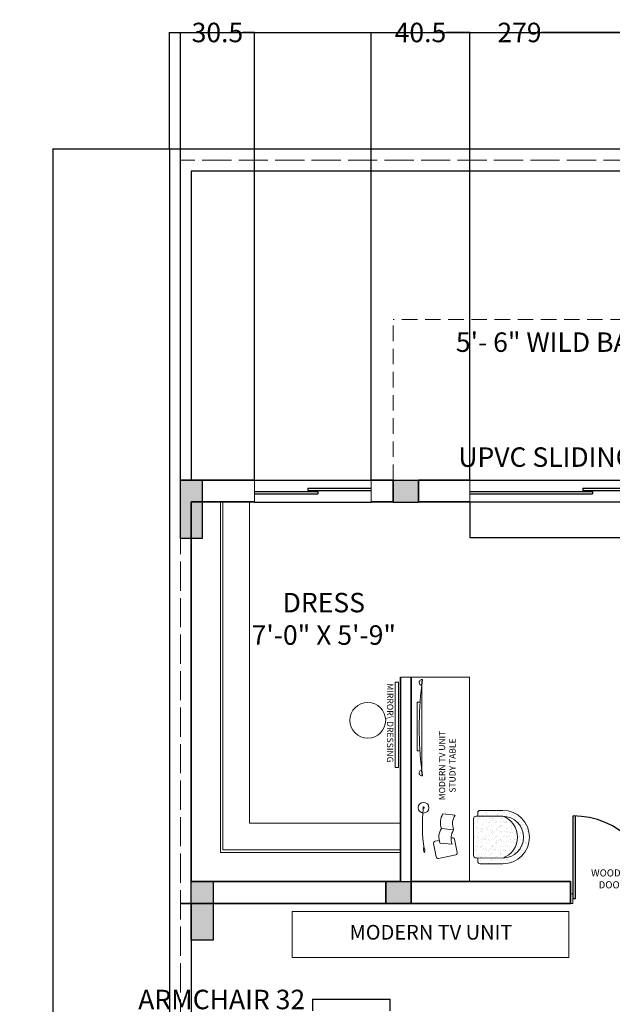
# Model space of a CAD drawing. Units: inches. Extents: x -48 to 50072, y 0 to 21068.
# Tile 54 of 75: x -48 to 196, y 819 to 1224. Entities that reach past the tile are written whole.
import ezdxf

# ---------------------------------------------------------------- set-up
doc = ezdxf.new("R2010")
doc.units = ezdxf.units.IN
doc.header["$MEASUREMENT"] = 0
doc.linetypes.add('ACAD_ISO02W100', pattern=[15, 12, -3])
doc.linetypes.add('HIDDEN', pattern=[9.525, 6.35, -3.175])
for name, color, linetype, lineweight in [('A-ANNO-DIMS', 2, 'Continuous', 18), ('A-ANNO-TEXT', 7, 'Continuous', 18), ('A-AREA-IDEN', 7, 'Continuous', 18), ('A-COLS', 1, 'Continuous', 35), ('A-DOOR', 4, 'Continuous', 18), ('A-EQPM', 8, 'Continuous', 18), ('A-FLOR-CASE', 9, 'Continuous', 18), ('A-FLOR-OVHD', 8, 'HIDDEN', 13), ('A-GLAZ', 4, 'Continuous', 18), ('A-WALL', 7, 'Continuous', 35), ('C-PROP', 7, 'Continuous', 25), ('C-PROP-REF', 32, 'ACAD_ISO02W100', 13), ('FURNITURE', 44, 'Continuous', 18)]:
    doc.layers.add(name, color=color, linetype=linetype, lineweight=lineweight)
doc.layers.add('Layer3', color=176, linetype='Continuous')
doc.styles.get("Standard").update_dxf_attribs({"font": 'arial.ttf'})
doc.dimstyles.get("Standard").update_dxf_attribs({"dimtxt": 8, "dimasz": 0.18, "dimexe": 0.18, "dimexo": 0.0625, "dimgap": 0.09, "dimtad": 0, "dimtih": 1, "dimtoh": 1, "dimdec": 1, "dimzin": 0, "dimdsep": 46, "dimlunit": 4, "dimtxsty": 'Standard', "dimblk": 'ARCHTICK', "dimcen": 0.09, "dimadec": 0, "dimazin": 0, "dimtfac": 1, "dimtdec": 1, "dimtofl": 0, "dimtmove": 0, "dimatfit": 3, "dimldrblk": 'ARCHTICK', "dimfxl": 1, "dimtolj": 1, "dimtzin": 0, "dimarcsym": 0})

# ---------------------------------------------------------------- blocks, each defined once
blk = doc.blocks.new('BKUHJKKUG')
at = {"layer": 'Defpoints'}
for p, q in [((179.52, 862.77), (179.52, 896.77)), ((180.52, 862.77), (180.52, 896.76)), ((179.52, 862.77), (180.52, 862.77))]:
    blk.add_line(p, q, dxfattribs=at)
blk.add_arc((179.52, 862.77), 34, 0, 90, dxfattribs=at)
at = {"insert": (190.84, 874.8), "char_height": 2.9183, "attachment_point": 1}
blk.add_mtext_dynamic_manual_height_columns('\\pxqc;WOODEN ^JDOOR', width=9.6242, gutter_width=14.59, heights=[0], dxfattribs=at)
blk = doc.blocks.new('khll')
at = {"layer": 'Defpoints'}
h = blk.add_hatch(color=256, dxfattribs=at)
h.dxf.hatch_style = 1
h.paths.add_polyline_path([(105.52, 1025.77), (116.02, 1025.77), (116.02, 1034.77), (105.52, 1034.77)])
for p, q in [((105.52, 1025.77), (105.52, 1034.77)), ((116.02, 1025.77), (116.02, 1034.77))]:
    blk.add_line(p, q)
for p, q in [((105.52, 1034.77), (116.02, 1034.77)), ((105.52, 1025.77), (116.02, 1025.77))]:
    blk.add_line(p, q, dxfattribs=at)
blk = doc.blocks.new('bnniku')
at = {"layer": 'Defpoints'}
h = blk.add_hatch(color=256, dxfattribs=at)
h.dxf.hatch_style = 1
h.paths.add_polyline_path([(767.55, 1114.04), (758.55, 1114.04), (758.55, 1090.04), (767.55, 1090.04)])
for p, q in [((758.55, 1114.04), (767.55, 1114.04)), ((758.55, 1090.04), (758.55, 1114.04)), ((767.55, 1114.04), (767.55, 1090.04)), ((767.55, 1090.04), (758.55, 1090.04))]:
    blk.add_line(p, q, dxfattribs=at)
blk = doc.blocks.new('windom')
for p, q in [((48.52, 1025.77), (48.52, 1034.77)), ((96.52, 1025.77), (96.52, 1034.77))]:
    blk.add_line(p, q)
at = {"layer": 'Defpoints'}
for p, q in [((48.52, 1030.07), (74.52, 1030.07)), ((48.52, 1029.07), (74.52, 1029.07)), ((70.52, 1031.47), (96.52, 1031.47)), ((70.52, 1031.47), (70.52, 1030.47)), ((70.52, 1030.47), (96.52, 1030.47)), ((74.52, 1030.07), (74.52, 1029.07))]:
    blk.add_line(p, q, dxfattribs=at)
at = {"layer": 'Layer3'}
for p, q in [((48.52, 1034.77), (96.52, 1034.77)), ((48.52, 1025.77), (96.52, 1025.77))]:
    blk.add_line(p, q, dxfattribs=at)
blk = doc.blocks.new('sliding')
blk.add_line((137.02, 1025.77), (137.02, 1034.77))
at = {"layer": 'Defpoints'}
for p, q in [((234.12, 1034.77), (234.12, 1025.77)), ((137.02, 1030.07), (187.57, 1030.07)), ((137.02, 1029.07), (187.57, 1029.07)), ((183.57, 1031.47), (234.12, 1031.47)), ((183.57, 1031.47), (183.57, 1030.47)), ((183.57, 1030.47), (234.12, 1030.47)), ((187.57, 1030.07), (187.57, 1029.07))]:
    blk.add_line(p, q, dxfattribs=at)
at = {"layer": 'Layer3'}
for p, q in [((137.02, 1034.77), (234.12, 1034.77)), ((234.12, 1025.77), (137.02, 1025.77))]:
    blk.add_line(p, q, dxfattribs=at)
blk = doc.blocks.new('CHAIR-STUDY')
for p, q in [((1.73, 20.94), (1.73, 19.57)), ((1.74, 20.38, 13.84), (1.74, 20.38, 13.84)), ((2.76, 21.97), (12.03, 21.96)), ((3.67, 21.9, 13.84), (3.67, 21.9, 13.84)), ((4.87, 21.05, 13.84), (4.87, 21.05, 13.84)), ((5.15, 21.3, 13.84), (5.15, 21.3, 13.84)), ((5.52, 20.9, 13.84), (5.52, 20.9, 13.84)), ((5.63, 20.39, 13.84), (5.63, 20.39, 13.84)), ((6.44, 21.95, 13.84), (6.44, 21.95, 13.84)), ((7.77, 21.75, 13.84), (7.77, 21.75, 13.84)), ((8.5, 21.68, 13.84), (8.5, 21.68, 13.84)), ((9.61, 20.34, 13.84), (9.61, 20.34, 13.84)), ((9.74, 21.52, 13.84), (9.74, 21.52, 13.84)), ((10.25, 20.89, 13.84), (10.25, 20.89, 13.84)), ((10.53, 21.41, 13.84), (10.53, 21.41, 13.84)), ((11.24, 21.36, 13.84), (11.24, 21.36, 13.84)), ((11.66, 21.77, 13.84), (11.66, 21.77, 13.84)), ((12.59, 21.14, 13.84), (12.59, 21.14, 13.84)), ((13.83, 20.98, 13.84), (13.83, 20.98, 13.84)), ((14.62, 20.87, 13.84), (14.62, 20.87, 13.84)), ((14.99, 20.88, 13.84), (14.99, 20.88, 13.84)), ((16.68, 20.6, 13.84), (16.68, 20.6, 13.84)), ((0.01, 18.54), (0, 3.44)), ((0.15, 18.84, 13.84), (0.15, 18.84, 13.84)), ((0.44, 16.98, 13.84), (0.44, 16.98, 13.84)), ((0.94, 18.74, 13.84), (0.94, 18.74, 13.84)), ((1.04, 19.57), (12.03, 19.56)), ((1.64, 17.45, 13.84), (1.64, 17.45, 13.84)), ((1.76, 18.19, 13.84), (1.76, 18.19, 13.84)), ((1.87, 18.57, 13.84), (1.87, 18.57, 13.84)), ((2.04, 18.45, 13.84), (2.04, 18.45, 13.84)), ((2.51, 18.98, 13.84), (2.51, 18.98, 13.84)), ((3.01, 18.47, 13.84), (3.01, 18.47, 13.84)), ((3.55, 19.84, 13.84), (3.55, 19.84, 13.84)), ((3.57, 18.97, 13.84), (3.57, 18.97, 13.84)), ((4.24, 18.3, 13.84), (4.24, 18.3, 13.84)), ((4.29, 17.09, 13.84), (4.29, 17.09, 13.84)), ((5.03, 18.2, 13.84), (5.03, 18.2, 13.84)), ((5.53, 17.47, 13.84), (5.53, 17.47, 13.84)), ((6.33, 16.86, 13.84), (6.33, 16.86, 13.84)), ((6.6, 18.56, 13.84), (6.6, 18.56, 13.84)), ((6.61, 17.12, 13.84), (6.61, 17.12, 13.84)), ((7.1, 17.93, 13.84), (7.1, 17.93, 13.84)), ((7.24, 18.97, 13.84), (7.24, 18.97, 13.84)), ((7.68, 18.82, 13.84), (7.68, 18.82, 13.84)), ((8.12, 18.5, 13.84), (8.12, 18.5, 13.84)), ((8.34, 17.77, 13.84), (8.34, 17.77, 13.84)), ((9.02, 17.09, 13.84), (9.02, 17.09, 13.84)), ((9.13, 17.66, 13.84), (9.13, 17.66, 13.84)), ((9.44, 19.71, 13.84), (9.44, 19.71, 13.84)), ((9.51, 17.42, 13.84), (9.51, 17.42, 13.84)), ((9.72, 19.97, 13.84), (9.72, 19.97, 13.84)), ((11.19, 17.39, 13.84), (11.19, 17.39, 13.84)), ((11.33, 18.56, 13.84), (11.33, 18.56, 13.84)), ((11.57, 18.84, 13.84), (11.57, 18.84, 13.84)), ((11.97, 18.96, 13.84), (11.97, 18.96, 13.84)), ((12.43, 17.23, 13.84), (12.43, 17.23, 13.84)), ((12.69, 17.17, 13.84), (12.69, 17.17, 13.84)), ((13.22, 17.12, 13.84), (13.22, 17.12, 13.84)), ((13.62, 17.27, 13.84), (13.62, 17.27, 13.84)), ((13.71, 20.2, 13.84), (13.71, 20.2, 13.84)), ((13.76, 17.08, 13.84), (13.76, 17.08, 13.84)), ((14.01, 18.38, 13.84), (14.01, 18.38, 13.84)), ((14.29, 18.64, 13.84), (14.29, 18.64, 13.84)), ((15.28, 16.85, 13.84), (15.28, 16.85, 13.84)), ((15.54, 18.79, 13.84), (15.54, 18.79, 13.84)), ((15.81, 20.02, 13.84), (15.81, 20.02, 13.84)), ((16.07, 18.55, 13.84), (16.07, 18.55, 13.84)), ((16.52, 16.69, 13.84), (16.52, 16.69, 13.84)), ((16.71, 18.96, 13.84), (16.71, 18.96, 13.84)), ((17.31, 16.58, 13.84), (17.31, 16.58, 13.84)), ((17.5, 17.29, 13.84), (17.5, 17.29, 13.84)), ((17.6, 20.21, 13.84), (17.6, 20.21, 13.84)), ((18.49, 17.07, 13.84), (18.49, 17.07, 13.84)), ((18.58, 17.05, 13.84), (18.58, 17.05, 13.84)), ((18.86, 17.3, 13.84), (18.86, 17.3, 13.84)), ((19.37, 16.31, 13.84), (19.37, 16.31, 13.84)), ((19.65, 18.64, 13.84), (19.65, 18.64, 13.84)), ((0.64, 14.77, 13.84), (0.64, 14.77, 13.84)), ((1.28, 15.17, 13.84), (1.28, 15.17, 13.84)), ((1.55, 14.52, 13.84), (1.55, 14.52, 13.84)), ((1.61, 14.72, 13.84), (1.61, 14.72, 13.84)), ((1.89, 12.79, 13.84), (1.89, 12.79, 13.84)), ((2.84, 14.55, 13.84), (2.84, 14.55, 13.84)), ((3.06, 13.29, 13.84), (3.06, 13.29, 13.84)), ((3.21, 14, 13.84), (3.21, 14, 13.84)), ((3.38, 13.11, 13.84), (3.38, 13.11, 13.84)), ((3.48, 16.04, 13.84), (3.48, 16.04, 13.84)), ((3.49, 14.26, 13.84), (3.49, 14.26, 13.84)), ((3.63, 14.45, 13.84), (3.63, 14.45, 13.84)), ((5.01, 15.65, 13.84), (5.01, 15.65, 13.84)), ((5.37, 14.76, 13.84), (5.37, 14.76, 13.84)), ((5.44, 14.54, 13.84), (5.44, 14.54, 13.84)), ((5.7, 14.18, 13.84), (5.7, 14.18, 13.84)), ((6.01, 15.17, 13.84), (6.01, 15.17, 13.84)), ((6.93, 14.01, 13.84), (6.93, 14.01, 13.84)), ((7.49, 12.96, 13.84), (7.49, 12.96, 13.84)), ((7.58, 15.89, 13.84), (7.58, 15.89, 13.84)), ((7.72, 13.91, 13.84), (7.72, 13.91, 13.84)), ((7.78, 12.67, 13.84), (7.78, 12.67, 13.84)), ((7.8, 13.28, 13.84), (7.8, 13.28, 13.84)), ((8.06, 12.93, 13.84), (8.06, 12.93, 13.84)), ((9.41, 14.49, 13.84), (9.41, 14.49, 13.84)), ((9.58, 14.31, 13.84), (9.58, 14.31, 13.84)), ((9.79, 13.64, 13.84), (9.79, 13.64, 13.84)), ((10.1, 14.75, 13.84), (10.1, 14.75, 13.84)), ((10.75, 15.16, 13.84), (10.75, 15.16, 13.84)), ((10.9, 15.52, 13.84), (10.9, 15.52, 13.84)), ((11.03, 13.48, 13.84), (11.03, 13.48, 13.84)), ((11.18, 15.78, 13.84), (11.18, 15.78, 13.84)), ((11.37, 12.98, 13.84), (11.37, 12.98, 13.84)), ((11.47, 15.91, 13.84), (11.47, 15.91, 13.84)), ((11.82, 13.37, 13.84), (11.82, 13.37, 13.84)), ((12.53, 13.27, 13.84), (12.53, 13.27, 13.84)), ((13.52, 14.34, 13.84), (13.52, 14.34, 13.84)), ((13.88, 13.1, 13.84), (13.88, 13.1, 13.84)), ((14.14, 12.98, 13.84), (14.14, 12.98, 13.84)), ((14.84, 14.74, 13.84), (14.84, 14.74, 13.84)), ((15.12, 12.94, 13.84), (15.12, 12.94, 13.84)), ((15.35, 12.93, 13.84), (15.35, 12.93, 13.84)), ((15.45, 15.86, 13.84), (15.45, 15.86, 13.84)), ((15.47, 14.19, 13.84), (15.47, 14.19, 13.84)), ((15.48, 15.15, 13.84), (15.48, 15.15, 13.84)), ((15.75, 14.45, 13.84), (15.75, 14.45, 13.84)), ((15.91, 12.83, 13.84), (15.91, 12.83, 13.84)), ((17.26, 15.83, 13.84), (17.26, 15.83, 13.84)), ((17.26, 13.26, 13.84), (17.26, 13.26, 13.84)), ((17.41, 14.36, 13.84), (17.41, 14.36, 13.84)), ((17.97, 12.56, 13.84), (17.97, 12.56, 13.84)), ((19.21, 12.4, 13.84), (19.21, 12.4, 13.84)), ((19.46, 12.78, 13.84), (19.46, 12.78, 13.84)), ((19.55, 15.71, 13.84), (19.55, 15.71, 13.84)), ((19.57, 14.73, 13.84), (19.57, 14.73, 13.84)), ((20, 12.29, 13.84), (20, 12.29, 13.84)), ((20.04, 12.86, 13.84), (20.04, 12.86, 13.84)), ((20.21, 15.14, 13.84), (20.21, 15.14, 13.84)), ((20.32, 13.11, 13.84), (20.32, 13.11, 13.84)), ((20.61, 16.15, 13.84), (20.61, 16.15, 13.84)), ((21.39, 14.31, 13.84), (21.39, 14.31, 13.84)), ((21.4, 16.05, 13.84), (21.4, 16.05, 13.84)), ((21.83, 14.5, 13.84), (21.83, 14.5, 13.84)), ((22, 13.25, 13.84), (22, 13.25, 13.84)), ((0.05, 11.37, 13.84), (0.05, 11.37, 13.84)), ((0.1, 11.15, 13.84), (0.1, 11.15, 13.84)), ((0.21, 10.96, 13.84), (0.21, 10.96, 13.84)), ((0.38, 11.41, 13.84), (0.38, 11.41, 13.84)), ((1.36, 8.66, 13.84), (1.36, 8.66, 13.84)), ((1.44, 10.8, 13.84), (1.44, 10.8, 13.84)), ((1.45, 11.59, 13.84), (1.45, 11.59, 13.84)), ((1.84, 9.48, 13.84), (1.84, 9.48, 13.84)), ((2.23, 10.7, 13.84), (2.23, 10.7, 13.84)), ((3.28, 10.18, 13.84), (3.28, 10.18, 13.84)), ((3.34, 8.6, 13.84), (3.34, 8.6, 13.84)), ((4.14, 10.95, 13.84), (4.14, 10.95, 13.84)), ((4.3, 10.43, 13.84), (4.3, 10.43, 13.84)), ((4.67, 9.81, 13.84), (4.67, 9.81, 13.84)), ((4.78, 11.36, 13.84), (4.78, 11.36, 13.84)), ((4.95, 10.07, 13.84), (4.95, 10.07, 13.84)), ((5.24, 8.68, 13.84), (5.24, 8.68, 13.84)), ((5.34, 11.61, 13.84), (5.34, 11.61, 13.84)), ((5.53, 10.26, 13.84), (5.53, 10.26, 13.84)), ((6.32, 10.16, 13.84), (6.32, 10.16, 13.84)), ((6.46, 11.46, 13.84), (6.46, 11.46, 13.84)), ((6.57, 9.47, 13.84), (6.57, 9.47, 13.84)), ((7.39, 10.04, 13.84), (7.39, 10.04, 13.84)), ((8.39, 9.89, 13.84), (8.39, 9.89, 13.84)), ((8.88, 10.94, 13.84), (8.88, 10.94, 13.84)), ((9.22, 8.63, 13.84), (9.22, 8.63, 13.84)), ((9.24, 8.48, 13.84), (9.24, 8.48, 13.84)), ((9.32, 11.56, 13.84), (9.32, 11.56, 13.84)), ((9.52, 11.35, 13.84), (9.52, 11.35, 13.84)), ((9.52, 8.74, 13.84), (9.52, 8.74, 13.84)), ((9.62, 9.72, 13.84), (9.62, 9.72, 13.84)), ((10.41, 9.62, 13.84), (10.41, 9.62, 13.84)), ((11.03, 10.12, 13.84), (11.03, 10.12, 13.84)), ((11.28, 10.05, 13.84), (11.28, 10.05, 13.84)), ((11.3, 9.46, 13.84), (11.3, 9.46, 13.84)), ((12.35, 11.34, 13.84), (12.35, 11.34, 13.84)), ((12.48, 9.35, 13.84), (12.48, 9.35, 13.84)), ((12.63, 11.59, 13.84), (12.63, 11.59, 13.84)), ((13.33, 8.48, 13.84), (13.33, 8.48, 13.84)), ((13.42, 11.41, 13.84), (13.42, 11.41, 13.84)), ((13.61, 10.93, 13.84), (13.61, 10.93, 13.84)), ((13.72, 9.19, 13.84), (13.72, 9.19, 13.84)), ((14.25, 11.34, 13.84), (14.25, 11.34, 13.84)), ((14.51, 9.08, 13.84), (14.51, 9.08, 13.84)), ((15.26, 10, 13.84), (15.26, 10, 13.84)), ((15.6, 8.79, 13.84), (15.6, 8.79, 13.84)), ((16.04, 9.46, 13.84), (16.04, 9.46, 13.84)), ((16.57, 8.81, 13.84), (16.57, 8.81, 13.84)), ((16.92, 10, 13.84), (16.92, 10, 13.84)), ((17.2, 10.26, 13.84), (17.2, 10.26, 13.84)), ((17.22, 8.5, 13.84), (17.22, 8.5, 13.84)), ((17.31, 11.43, 13.84), (17.31, 11.43, 13.84)), ((17.81, 8.65, 13.84), (17.81, 8.65, 13.84)), ((18.34, 10.93, 13.84), (18.34, 10.93, 13.84)), ((18.6, 8.54, 13.84), (18.6, 8.54, 13.84)), ((18.71, 11.64, 13.84), (18.71, 11.64, 13.84)), ((18.99, 11.33, 13.84), (18.99, 11.33, 13.84)), ((19.36, 9.86, 13.84), (19.36, 9.86, 13.84)), ((20.66, 8.27, 13.84), (20.66, 8.27, 13.84)), ((20.77, 9.45, 13.84), (20.77, 9.45, 13.84)), ((21.2, 8.45, 13.84), (21.2, 8.45, 13.84)), ((21.29, 11.38, 13.84), (21.29, 11.38, 13.84)), ((21.49, 8.67, 13.84), (21.49, 8.67, 13.84)), ((21.77, 8.92, 13.84), (21.77, 8.92, 13.84)), ((21.9, 8.11, 13.84), (21.9, 8.11, 13.84)), ((22.06, 12.02, 13.84), (22.06, 12.02, 13.84)), ((0.04, 7.05, 13.84), (0.04, 7.05, 13.84)), ((0.23, 5.75, 13.84), (0.23, 5.75, 13.84)), ((0.61, 5.68, 13.84), (0.61, 5.68, 13.84)), ((0.83, 6.95, 13.84), (0.83, 6.95, 13.84)), ((1.26, 5.73, 13.84), (1.26, 5.73, 13.84)), ((1.55, 6.96, 13.84), (1.55, 6.96, 13.84)), ((1.83, 7.22, 13.84), (1.83, 7.22, 13.84)), ((2.9, 6.68, 13.84), (2.9, 6.68, 13.84)), ((2.92, 7.15, 13.84), (2.92, 7.15, 13.84)), ((3.09, 4.33, 13.84), (3.09, 4.33, 13.84)), ((3.19, 7.25, 13.84), (3.19, 7.25, 13.84)), ((3.56, 7.55, 13.84), (3.56, 7.55, 13.84)), ((4.13, 6.51, 13.84), (4.13, 6.51, 13.84)), ((4.8, 4.41, 13.84), (4.8, 4.41, 13.84)), ((4.92, 6.41, 13.84), (4.92, 6.41, 13.84)), ((5.15, 5.75, 13.84), (5.15, 5.75, 13.84)), ((5.34, 5.67, 13.84), (5.34, 5.67, 13.84)), ((6.12, 5.63, 13.84), (6.12, 5.63, 13.84)), ((6.4, 5.88, 13.84), (6.4, 5.88, 13.84)), ((6.99, 6.14, 13.84), (6.99, 6.14, 13.84)), ((7.2, 4.18, 13.84), (7.2, 4.18, 13.84)), ((7.29, 7.11, 13.84), (7.29, 7.11, 13.84)), ((7.65, 7.14, 13.84), (7.65, 7.14, 13.84)), ((7.91, 7.27, 13.84), (7.91, 7.27, 13.84)), ((8.22, 5.97, 13.84), (8.22, 5.97, 13.84)), ((8.29, 7.55, 13.84), (8.29, 7.55, 13.84)), ((9.01, 5.87, 13.84), (9.01, 5.87, 13.84)), ((9.13, 5.7, 13.84), (9.13, 5.7, 13.84)), ((10.08, 5.66, 13.84), (10.08, 5.66, 13.84)), ((10.69, 4.29, 13.84), (10.69, 4.29, 13.84)), ((10.97, 4.55, 13.84), (10.97, 4.55, 13.84)), ((11.08, 5.6, 13.84), (11.08, 5.6, 13.84)), ((11.09, 4.2, 13.84), (11.09, 4.2, 13.84)), ((11.18, 7.13, 13.84), (11.18, 7.13, 13.84)), ((12.31, 5.44, 13.84), (12.31, 5.44, 13.84)), ((12.38, 7.13, 13.84), (12.38, 7.13, 13.84)), ((12.48, 5.93, 13.84), (12.48, 5.93, 13.84)), ((13.02, 7.54, 13.84), (13.02, 7.54, 13.84)), ((13.1, 5.33, 13.84), (13.1, 5.33, 13.84)), ((13.23, 5.55, 13.84), (13.23, 5.55, 13.84)), ((13.81, 7.15, 13.84), (13.81, 7.15, 13.84)), ((14.09, 7.4, 13.84), (14.09, 7.4, 13.84)), ((14.81, 5.65, 13.84), (14.81, 5.65, 13.84)), ((15.07, 4.15, 13.84), (15.07, 4.15, 13.84)), ((15.16, 7.07, 13.84), (15.16, 7.07, 13.84)), ((15.17, 5.06, 13.84), (15.17, 5.06, 13.84)), ((16.41, 4.9, 13.84), (16.41, 4.9, 13.84)), ((17.05, 4.6, 13.84), (17.05, 4.6, 13.84)), ((17.12, 7.12, 13.84), (17.12, 7.12, 13.84)), ((17.12, 5.57, 13.84), (17.12, 5.57, 13.84)), ((17.2, 4.79, 13.84), (17.2, 4.79, 13.84)), ((17.76, 7.53, 13.84), (17.76, 7.53, 13.84)), ((18.37, 5.81, 13.84), (18.37, 5.81, 13.84)), ((18.65, 6.07, 13.84), (18.65, 6.07, 13.84)), ((19.26, 4.52, 13.84), (19.26, 4.52, 13.84)), ((19.27, 6.93, 13.84), (19.27, 6.93, 13.84)), ((19.54, 5.64, 13.84), (19.54, 5.64, 13.84)), ((20.17, 7.46, 13.84), (20.17, 7.46, 13.84)), ((20.5, 4.36, 13.84), (20.5, 4.36, 13.84)), ((21.1, 5.52, 13.84), (21.1, 5.52, 13.84)), ((21.85, 7.11, 13.84), (21.85, 7.11, 13.84)), ((1.03, 2.41), (12.01, 2.4)), ((1.16, 2.8, 13.84), (1.16, 2.8, 13.84)), ((1.49, 2.92, 13.84), (1.49, 2.92, 13.84)), ((1.69, 3.34, 13.84), (1.69, 3.34, 13.84)), ((1.72, 2.41), (1.71, 1.04)), ((2.33, 3.75, 13.84), (2.33, 3.75, 13.84)), ((2.73, 2.76, 13.84), (2.73, 2.76, 13.84)), ((2.74, 0.01), (12.01, 0)), ((3, 1.4, 13.84), (3, 1.4, 13.84)), ((3.01, 2.77, 13.84), (3.01, 2.77, 13.84)), ((3.29, 3.03, 13.84), (3.29, 3.03, 13.84)), ((3.52, 2.66, 13.84), (3.52, 2.66, 13.84)), ((4.11, 1.86, 13.84), (4.11, 1.86, 13.84)), ((5.05, 2.82, 13.84), (5.05, 2.82, 13.84)), ((5.59, 2.39, 13.84), (5.59, 2.39, 13.84)), ((6.25, 0.23, 13.84), (6.25, 0.23, 13.84)), ((6.42, 3.33, 13.84), (6.42, 3.33, 13.84)), ((6.82, 2.22, 13.84), (6.82, 2.22, 13.84)), ((7.06, 3.74, 13.84), (7.06, 3.74, 13.84)), ((7.1, 1.25, 13.84), (7.1, 1.25, 13.84)), ((7.57, 1.44, 13.84), (7.57, 1.44, 13.84)), ((7.61, 2.12, 13.84), (7.61, 2.12, 13.84)), ((7.85, 1.69, 13.84), (7.85, 1.69, 13.84)), ((8.85, 1.85, 13.84), (8.85, 1.85, 13.84)), ((9.03, 2.77, 13.84), (9.03, 2.77, 13.84)), ((9.37, 3.08, 13.84), (9.37, 3.08, 13.84)), ((9.68, 1.85, 13.84), (9.68, 1.85, 13.84)), ((10.91, 1.68, 13.84), (10.91, 1.68, 13.84)), ((10.99, 1.27, 13.84), (10.99, 1.27, 13.84)), ((11.16, 3.32, 13.84), (11.16, 3.32, 13.84)), ((11.7, 1.58, 13.84), (11.7, 1.58, 13.84)), ((11.8, 3.73, 13.84), (11.8, 3.73, 13.84)), ((12.14, 0.1, 13.84), (12.14, 0.1, 13.84)), ((12.42, 0.36, 13.84), (12.42, 0.36, 13.84)), ((13.14, 2.62, 13.84), (13.14, 2.62, 13.84)), ((13.58, 1.84, 13.84), (13.58, 1.84, 13.84)), ((13.77, 1.31, 13.84), (13.77, 1.31, 13.84)), ((13.94, 1.75, 13.84), (13.94, 1.75, 13.84)), ((14.97, 1.22, 13.84), (14.97, 1.22, 13.84)), ((15, 1.15, 13.84), (15, 1.15, 13.84)), ((15.26, 2.96, 13.84), (15.26, 2.96, 13.84)), ((15.54, 3.21, 13.84), (15.54, 3.21, 13.84)), ((15.8, 1.04, 13.84), (15.8, 1.04, 13.84)), ((15.89, 3.31, 13.84), (15.89, 3.31, 13.84)), ((16.53, 3.72, 13.84), (16.53, 3.72, 13.84)), ((17.02, 2.64, 13.84), (17.02, 2.64, 13.84)), ((19.17, 4, 13.84), (19.17, 4, 13.84))]:
    blk.add_line(p, q)
for centre, radius, start, end in [((2.76, 20.94), 1.03, 89.9486, 179.9486), ((12.02, 10.98), 10.98, 359.9486, 89.9486), ((1.04, 18.54), 1.03, 89.9486, 179.9486), ((9.02, 10.98), 9.09, 289.2386, 70.6585), ((12.02, 10.98), 8.58, 359.9486, 89.9486), ((12.02, 10.98), 10.98, 269.9486, 359.9486), ((12.02, 10.98), 8.58, 269.9486, 359.9486), ((1.03, 3.44), 1.03, 179.9486, 269.9486), ((2.74, 1.04), 1.03, 179.9486, 269.9486)]:
    blk.add_arc(centre, radius, start, end)
blk = doc.blocks.new('DESK-ACCESSORIES')
for p, q in [((10.18, 18.3), (15.19, 17.78)), ((9.56, 12.3), (14.56, 11.78)), ((13.5, 8.38), (14.02, 8.49)), ((7.43, 0.64), (6.33, 6.13)), ((6.96, 7.08), (8.64, 7.41)), ((13.94, 5.81), (8.93, 6.33)), ((14.96, 7.86), (16.06, 2.37)), ((15.43, 1.43), (8.37, 0.02))]:
    blk.add_line(p, q)
for centre, radius, start, end in [((2.2, 20.84), 2.2, 90, 270), ((63.85, 13.23), 62.16, 173.4513, 188.6305), ((2.2, 20.84), 0.3, 90, 270), ((2.2, 20.84), 2.2, 270, 90), ((2.2, 20.84), 0.3, 270, 90), ((15.87, 14.66), 6.76, 147.37, 200.7442), ((20.88, 14.14), 6.76, 147.37, 200.7442), ((15.03, 8.7), 6.54, 146.9045, 201.2097), ((20.04, 8.18), 6.54, 146.9045, 201.2097), ((14.18, 7.7), 0.8, 11.3025, 101.3025), ((4, 3.71), 1.82, 157.356, 216.9378), ((2.33, 4.39), 0.12, 90, 270), ((0.87, 3.31), 1.82, 337.356, 36.9378), ((2.33, 4.39), 0.12, 270, 90), ((7.12, 6.29), 0.8, 101.3025, 191.3025), ((2.54, 2.6), 0.12, 90, 270), ((2.54, 2.6), 0.12, 270, 90), ((8.21, 0.8), 0.8, 191.3025, 281.3025), ((15.27, 2.21), 0.8, 281.3025, 11.3025)]:
    blk.add_arc(centre, radius, start, end)
blk = doc.blocks.new('DISPLAY-FLAT-PANEL')
for p, q in [((1.73, 37.17), (2.01, 39.54)), ((1.83, 37.19), (2.11, 39.53)), ((1.83, 2.35), (1.83, 37.19)), ((1.83, 37.19), (1.83, 37.19)), ((1.2, 30.3), (0, 30.3)), ((0, 30.3), (0, 10.23)), ((0, 10.23), (1.13, 10.23)), ((1.73, 2.37), (2.01, 0)), ((1.83, 2.35), (2.11, 0.01))]:
    blk.add_line(p, q)
for centre, radius, start, end in [((1.97, 38.34), 1.2, 83.3215, 263.5313), ((153.03, 19.77), 152.2, 173.4285, 186.5715), ((1.97, 1.2), 1.2, 96.4687, 276.6785)]:
    blk.add_arc(centre, radius, start, end)
blk = doc.blocks.new('WARDROBE-L-RETURN')
for p, q in [((0, 144), (0, 0)), ((1, 144), (1, 1)), ((12, 144), (12, 12)), ((74, 12), (12, 12)), ((74, 1), (1, 1)), ((74, 0), (0, 0))]:
    blk.add_line(p, q)
blk = doc.blocks.new('_ArchTick')
at = {"color": 0, "linetype": 'ByBlock', "const_width": 0.15}
blk.add_lwpolyline([(-0.5, -0.5), (0.5, 0.5)], dxfattribs=at)
blk = doc.blocks.new('*D62')
at = {"layer": 'A-ANNO-DIMS', "color": 0, "lineweight": -2, "transparency": 16777216}
for p, q in [((137.02, 1025.71), (137.02, 1011.03)), ((234.12, 1025.71), (234.12, 1011.03)), ((137.02, 1011.21), (234.12, 1011.21)), ((234.12, 1011.21), (234.3, 1011.21))]:
    blk.add_line(p, q, dxfattribs=at)
at = {"layer": 'Defpoints', "color": 0, "transparency": 16777216}
for p in [(137.02, 1025.77), (234.12, 1025.77), (234.12, 1011.21)]:
    blk.add_point(p, dxfattribs=at)
at = {"layer": 'A-ANNO-DIMS', "color": 0, "lineweight": -2, "transparency": 16777216, "xscale": 0.18, "yscale": 0.18, "zscale": 0.18, "rotation": 180}
blk.add_blockref('_ArchTick', (137.02, 1011.21), dxfattribs=at)
at = {"layer": 'A-ANNO-DIMS', "color": 0, "lineweight": -2, "transparency": 16777216, "xscale": 0.18, "yscale": 0.18, "zscale": 0.18}
blk.add_blockref('_ArchTick', (234.12, 1011.21), dxfattribs=at)
at = {"layer": 'A-ANNO-DIMS', "color": 0, "transparency": 16777216, "insert": (301.34, 1011.21), "char_height": 8, "attachment_point": 5}
blk.add_mtext('\\A1;SLIDING DOOR B 97 TYP.', dxfattribs=at)
blk = doc.blocks.new('*D110')
at = {"layer": 'A-ANNO-DIMS', "color": 0, "lineweight": -2, "transparency": 16777216}
for p, q in [((72.57, 816.64), (72.57, 821.52)), ((104.32, 816.64), (104.32, 821.52)), ((72.57, 821.34), (72.39, 821.34)), ((104.32, 821.34), (72.57, 821.34))]:
    blk.add_line(p, q, dxfattribs=at)
at = {"layer": 'Defpoints', "color": 0, "transparency": 16777216}
for p in [(72.57, 821.34), (72.57, 816.58), (104.32, 816.58)]:
    blk.add_point(p, dxfattribs=at)
at = {"layer": 'A-ANNO-DIMS', "color": 0, "lineweight": -2, "transparency": 16777216, "xscale": 0.18, "yscale": 0.18, "zscale": 0.18, "rotation": 180}
blk.add_blockref('_ArchTick', (72.57, 821.34), dxfattribs=at)
at = {"layer": 'A-ANNO-DIMS', "color": 0, "lineweight": -2, "transparency": 16777216, "xscale": 0.18, "yscale": 0.18, "zscale": 0.18}
blk.add_blockref('_ArchTick', (104.32, 821.34), dxfattribs=at)
at = {"layer": 'A-ANNO-DIMS', "color": 0, "transparency": 16777216, "insert": (35.02, 821.34), "char_height": 8, "attachment_point": 5}
blk.add_mtext('\\A1;ARMCHAIR 32', dxfattribs=at)
blk = doc.blocks.new('*D112')
at = {"layer": 'A-ANNO-DIMS', "color": 0, "lineweight": -2, "transparency": 16777216}
for p, q in [((13.52, 1170.84), (13.52, 1218.9)), ((13.52, 1218.72), (274.6, 1218.72)), ((553.52, 1218.72), (292.43, 1218.72)), ((553.52, 1170.84), (553.52, 1218.9))]:
    blk.add_line(p, q, dxfattribs=at)
at = {"layer": 'Defpoints', "color": 0, "transparency": 16777216}
for p in [(553.52, 1218.72), (13.52, 1170.77), (553.52, 1170.77)]:
    blk.add_point(p, dxfattribs=at)
at = {"layer": 'A-ANNO-DIMS', "color": 0, "lineweight": -2, "transparency": 16777216, "xscale": 0.18, "yscale": 0.18, "zscale": 0.18, "rotation": 180}
blk.add_blockref('_ArchTick', (13.52, 1218.72), dxfattribs=at)
at = {"layer": 'A-ANNO-DIMS', "color": 0, "lineweight": -2, "transparency": 16777216, "xscale": 0.18, "yscale": 0.18, "zscale": 0.18}
blk.add_blockref('_ArchTick', (553.52, 1218.72), dxfattribs=at)
at = {"layer": 'A-ANNO-DIMS', "color": 0, "transparency": 16777216, "insert": (283.52, 1218.72), "char_height": 8, "attachment_point": 5}
blk.add_mtext('\\A1;540', dxfattribs=at)
blk = doc.blocks.new('*D113')
at = {"layer": 'A-ANNO-DIMS', "color": 0, "lineweight": -2, "transparency": 16777216}
for p, q in [((13.45, 1170.77), (-34.61, 1170.77)), ((-34.43, 1170.77), (-34.43, 696.6)), ((-34.43, 214.07), (-34.43, 688.25)), ((13.45, 214.07), (-34.61, 214.07))]:
    blk.add_line(p, q, dxfattribs=at)
at = {"layer": 'Defpoints', "color": 0, "transparency": 16777216}
for p in [(-34.43, 1170.77), (13.52, 1170.77), (13.52, 214.07)]:
    blk.add_point(p, dxfattribs=at)
at = {"layer": 'A-ANNO-DIMS', "color": 0, "lineweight": -2, "transparency": 16777216, "xscale": 0.18, "yscale": 0.18, "zscale": 0.18}
for p, rotation in [((-34.43, 1170.77), 90), ((-34.43, 214.07), 270)]:
    blk.add_blockref('_ArchTick', p, dxfattribs=dict(at, rotation=rotation))
at = {"layer": 'A-ANNO-DIMS', "color": 0, "transparency": 16777216, "insert": (-34.43, 692.42), "char_height": 8, "attachment_point": 5}
blk.add_mtext('\\A1;956.7', dxfattribs=at)
blk = doc.blocks.new('*D123')
at = {"layer": 'A-ANNO-DIMS', "color": 0, "lineweight": -2, "transparency": 16777216}
for p, q in [((18.02, 1034.84), (18.02, 1218.9)), ((18.02, 1218.72), (148.51, 1218.72)), ((297.02, 1218.72), (166.52, 1218.72)), ((297.02, 1034.84), (297.02, 1218.9))]:
    blk.add_line(p, q, dxfattribs=at)
at = {"layer": 'Defpoints', "color": 0, "transparency": 16777216}
for p in [(297.02, 1218.72), (18.02, 1034.77), (297.02, 1034.77)]:
    blk.add_point(p, dxfattribs=at)
at = {"layer": 'A-ANNO-DIMS', "color": 0, "lineweight": -2, "transparency": 16777216, "xscale": 0.18, "yscale": 0.18, "zscale": 0.18, "rotation": 180}
blk.add_blockref('_ArchTick', (18.02, 1218.72), dxfattribs=at)
at = {"layer": 'A-ANNO-DIMS', "color": 0, "lineweight": -2, "transparency": 16777216, "xscale": 0.18, "yscale": 0.18, "zscale": 0.18}
blk.add_blockref('_ArchTick', (297.02, 1218.72), dxfattribs=at)
at = {"layer": 'A-ANNO-DIMS', "color": 0, "transparency": 16777216, "insert": (157.52, 1218.72), "char_height": 8, "attachment_point": 5}
blk.add_mtext('\\A1;279', dxfattribs=at)
blk = doc.blocks.new('*D125')
at = {"layer": 'A-ANNO-DIMS', "color": 0, "lineweight": -2, "transparency": 16777216}
for p, q in [((18.02, 1034.84), (18.02, 1218.9)), ((18.02, 1218.72), (22.76, 1218.72)), ((48.52, 1218.72), (43.77, 1218.72)), ((48.52, 1034.84), (48.52, 1218.9))]:
    blk.add_line(p, q, dxfattribs=at)
at = {"layer": 'Defpoints', "color": 0, "transparency": 16777216}
for p in [(48.52, 1218.72), (18.02, 1034.77), (48.52, 1034.77)]:
    blk.add_point(p, dxfattribs=at)
at = {"layer": 'A-ANNO-DIMS', "color": 0, "lineweight": -2, "transparency": 16777216, "xscale": 0.18, "yscale": 0.18, "zscale": 0.18, "rotation": 180}
blk.add_blockref('_ArchTick', (18.02, 1218.72), dxfattribs=at)
at = {"layer": 'A-ANNO-DIMS', "color": 0, "lineweight": -2, "transparency": 16777216, "xscale": 0.18, "yscale": 0.18, "zscale": 0.18}
blk.add_blockref('_ArchTick', (48.52, 1218.72), dxfattribs=at)
at = {"layer": 'A-ANNO-DIMS', "color": 0, "transparency": 16777216, "insert": (33.27, 1218.72), "char_height": 8, "attachment_point": 5}
blk.add_mtext('\\A1;30.5', dxfattribs=at)
blk = doc.blocks.new('*D126')
at = {"layer": 'A-ANNO-DIMS', "color": 0, "lineweight": -2, "transparency": 16777216}
for p, q in [((96.52, 1034.84), (96.52, 1218.9)), ((96.52, 1218.72), (106.1, 1218.72)), ((137.02, 1218.72), (127.44, 1218.72)), ((137.02, 1034.84), (137.02, 1218.9))]:
    blk.add_line(p, q, dxfattribs=at)
at = {"layer": 'Defpoints', "color": 0, "transparency": 16777216}
for p in [(137.02, 1218.72), (96.52, 1034.77), (137.02, 1034.77)]:
    blk.add_point(p, dxfattribs=at)
at = {"layer": 'A-ANNO-DIMS', "color": 0, "lineweight": -2, "transparency": 16777216, "xscale": 0.18, "yscale": 0.18, "zscale": 0.18, "rotation": 180}
blk.add_blockref('_ArchTick', (96.52, 1218.72), dxfattribs=at)
at = {"layer": 'A-ANNO-DIMS', "color": 0, "lineweight": -2, "transparency": 16777216, "xscale": 0.18, "yscale": 0.18, "zscale": 0.18}
blk.add_blockref('_ArchTick', (137.02, 1218.72), dxfattribs=at)
at = {"layer": 'A-ANNO-DIMS', "color": 0, "transparency": 16777216, "insert": (116.77, 1218.72), "char_height": 8, "attachment_point": 5}
blk.add_mtext('\\A1;40.5', dxfattribs=at)

msp = doc.modelspace()

# ---------------------------------------------------------------- linework, layer by layer
at = {"layer": 'A-DOOR'}
for p, q in [((178.517, 864.775), (179.517, 864.775)), ((179.517, 864.775), (179.517, 860.775)), ((178.517, 860.775), (179.517, 860.775))]:
    msp.add_line(p, q, dxfattribs=at)
at = {"layer": 'A-FLOR-CASE'}
for p, q in [((137.017, 953.775), (108.517, 953.775)), ((137.017, 869.775), (137.017, 953.775))]:
    msp.add_line(p, q, dxfattribs=at)
msp.add_lwpolyline([(63.985, 857.464), (177.828, 857.464), (177.828, 838.627), (63.985, 838.627)], close=True, dxfattribs=at)
at = {"layer": 'A-FLOR-OVHD'}
for p in [(105.517, 1034.775), (306.017, 1100.775)]:
    msp.add_line(p, (105.517, 1100.775), dxfattribs=at)
at = {"layer": 'A-WALL'}
for p, q in [((48.517, 1034.775), (18.017, 1034.775)), ((105.517, 1034.775), (96.517, 1034.775)), ((137.017, 1034.775), (116.017, 1034.775)), ((22.517, 1025.775), (22.517, 869.775)), ((48.517, 1025.775), (22.517, 1025.775)), ((105.517, 1025.775), (96.517, 1025.775)), ((137.017, 1025.775), (116.017, 1025.775)), ((108.517, 869.775), (108.517, 953.775)), ((113.017, 869.775), (113.017, 953.775)), ((108.517, 869.775), (22.517, 869.775)), ((178.517, 869.775), (113.017, 869.775)), ((178.517, 869.775), (178.517, 860.775)), ((178.517, 860.775), (18.017, 860.775))]:
    msp.add_line(p, q, dxfattribs=at)
at = {"layer": 'C-PROP'}
for p, q in [((553.517, 1170.775), (13.517, 1170.775)), ((13.517, 1170.775), (13.517, 214.075)), ((544.517, 1161.775), (22.517, 1161.775)), ((22.517, 1161.775), (22.517, 1034.775)), ((22.517, 860.775), (22.517, 223.075))]:
    msp.add_line(p, q, dxfattribs=at)
at = {"layer": 'C-PROP-REF'}
for p, q in [((18.017, 1166.275), (18.017, 214.075)), ((549.017, 1166.275), (18.017, 1166.275))]:
    msp.add_line(p, q, dxfattribs=at)
at = {"layer": 'FURNITURE'}
msp.add_lwpolyline([(106.381, 951.715), (107.686, 951.715), (107.686, 916.636), (106.381, 916.636)], close=True, dxfattribs=at)
msp.add_circle((95.121, 936.057), 7.352, dxfattribs=at)

# ---------------------------------------------------------------- block references
at = {"layer": 'A-COLS'}
for name, p in [('bnniku', (-740.534, -79.262)), ('khll', (0, 0)), ('bnniku', (-736.034, -244.262)), ('khll', (-3, -165))]:
    msp.add_blockref(name, p, dxfattribs=at)
at = {"layer": 'A-DOOR'}
for name in ['sliding', 'BKUHJKKUG']:
    msp.add_blockref(name, (0, 0), dxfattribs=at)
at = {"layer": 'A-EQPM'}
msp.add_blockref('DISPLAY-FLAT-PANEL', (115.462, 913.243), dxfattribs=at)
at = {"layer": 'A-FLOR-CASE'}
msp.add_blockref('WARDROBE-L-RETURN', (34.517, 881.775), dxfattribs=at)
at = {"layer": 'A-GLAZ'}
msp.add_blockref('windom', (0, 0), dxfattribs=at)
at = {"layer": 'FURNITURE'}
for name, p in [('DESK-ACCESSORIES', (115.863, 879.311)), ('CHAIR-STUDY', (138.611, 877.076))]:
    msp.add_blockref(name, p, dxfattribs=at)

# ---------------------------------------------------------------- texts
at = {"layer": 'A-ANNO-TEXT', "attachment_point": 1}
for s, width, gutter_width, insert, char_height in [('5\'- 6" WILD BALCONY ADOVE ', 220.65422, 40, (131.359, 1095.463), 8), ('UPVC SLIDING DOOR ', 126.59735, 40, (132.36, 1048.223), 8), ('MODERN TV UNIT ', 155.64677, 30.136, (87.603, 851.974), 6.02726)]:
    msp.add_mtext_dynamic_manual_height_columns(s, width=width, gutter_width=gutter_width, heights=[0], dxfattribs=dict(at, insert=insert, char_height=char_height))
for s, width, gutter_width, insert, char_height, rotation in [('MIRROR\\\\ DRESSING', 49.25606, 13.012, (105.599, 951.27), 2.60237, 270), ('\\pxqc;MODERN TV UNIT ^JSTUDY TABLE ', 105.60938, 12.855, (124.372, 864.676), 2.57094, 90)]:
    msp.add_mtext_dynamic_manual_height_columns(s, width=width, gutter_width=gutter_width, heights=[0], dxfattribs=dict(at, insert=insert, char_height=char_height, rotation=rotation))
at = {"layer": 'A-AREA-IDEN', "insert": (12.997, 988.433), "char_height": 8, "attachment_point": 1}
msp.add_mtext_dynamic_manual_height_columns('\\pxqc;DRESS^J7\'-0" X 5\'-9"', width=128.05681, gutter_width=40, heights=[0], dxfattribs=at)

# ---------------------------------------------------------------- dimensions: what is measured, and where the dimension line sits
at = {"layer": 'A-ANNO-DIMS'}
for base, p1, p2, override, picture, middle in [((553.517, 1218.725), (13.517, 1170.775), (553.517, 1170.775), {"dimdec": 0, "dimlfac": 1, "dimrnd": 0, "dimzin": 0, "dimdsep": 46, "dimlunit": 2}, '*D112', (283.517, 1218.725)), ((297.017, 1218.725), (18.017, 1034.775), (297.017, 1034.775), {"dimdec": 0, "dimlfac": 1, "dimrnd": 0, "dimzin": 0, "dimdsep": 46, "dimlunit": 2}, '*D123', (157.517, 1218.725)), ((48.517, 1218.725), (18.017, 1034.775), (48.517, 1034.775), {"dimdec": 1, "dimlfac": 1, "dimrnd": 0, "dimzin": 0, "dimdsep": 46, "dimlunit": 2}, '*D125', (33.267, 1218.725)), ((137.017, 1218.725), (96.517, 1034.775), (137.017, 1034.775), {"dimdec": 1, "dimlfac": 1, "dimrnd": 0, "dimzin": 0, "dimdsep": 46, "dimlunit": 2}, '*D126', (116.767, 1218.725))]:
    dim = msp.add_linear_dim(base=base, p1=p1, p2=p2, dimstyle='Standard', override=override, dxfattribs=at)
    dim.commit()
    dim.dimension.update_dxf_attribs({"geometry": picture, "text_midpoint": middle})
dim = msp.add_linear_dim(base=(-34.433, 1170.775), p1=(13.517, 214.075), p2=(13.517, 1170.775), angle=90, dimstyle='Standard', override={"dimdec": 1, "dimlfac": 1, "dimrnd": 0, "dimzin": 0, "dimdsep": 46, "dimlunit": 2}, dxfattribs=at)
dim.commit()
dim.dimension.update_dxf_attribs({"geometry": '*D113', "text_midpoint": (-34.433, 692.425)})
dim = msp.add_linear_dim(base=(234.116, 1011.21), p1=(137.017, 1025.775), p2=(234.116, 1025.775), text='SLIDING DOOR B <> TYP.', dimstyle='Standard', override={"dimdec": 0, "dimlfac": 1, "dimrnd": 0, "dimzin": 0, "dimdsep": 46, "dimlunit": 2}, dxfattribs=at)
dim.commit()
dim.dimension.update_dxf_attribs({"geometry": '*D62', "text_midpoint": (301.343, 1011.21)})
dim = msp.add_linear_dim(base=(72.572, 821.343), p1=(104.323, 816.58), p2=(72.572, 816.58), angle=180, text='ARMCHAIR <>', dimstyle='Standard', override={"dimdec": 0, "dimlfac": 1, "dimrnd": 0, "dimzin": 0, "dimdsep": 46, "dimlunit": 2}, dxfattribs=at)
dim.commit()
dim.dimension.update_dxf_attribs({"geometry": '*D110', "text_midpoint": (35.025, 821.343)})

doc.saveas('drawing.dxf')
